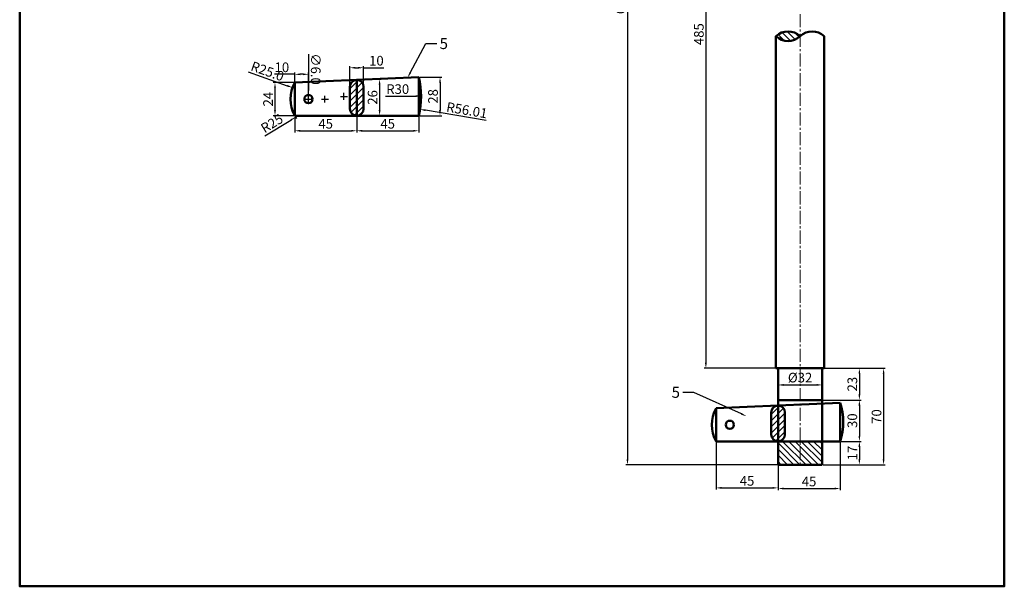
# Model space of a CAD drawing. Units: millimetres. Extents: x -21 to 693, y -570 to 295.
# Tile 1 of 7: x -21 to 693, y -570 to -159. Entities that reach past the tile are written whole.
import ezdxf
from ezdxf import colors
from ezdxf.entities.mleader import LeaderData, LeaderLine
from ezdxf.math import Vec2, Vec3

# ---------------------------------------------------------------- set-up
doc = ezdxf.new("R2010")
doc.units = ezdxf.units.MM
doc.header["$LTSCALE"] = 0.5
doc.linetypes.add('CENTER2', pattern=[28.575, 19.05, -3.175, 3.175, -3.175])
for name, color, linetype, lineweight in [('M-CNTR', 1, 'CENTER2', 18), ('M-DIMS', 2, 'Continuous', 25), ('M-HATC', 8, 'Continuous', 18), ('M-OUTL', 7, 'Continuous', 50), ('M-TEXT', 3, 'Continuous', 25), ('M-TTLB', 7, 'Continuous', 50)]:
    doc.layers.add(name, color=color, linetype=linetype, lineweight=lineweight)
doc.styles.get("Standard").update_dxf_attribs({"font": 'arial.ttf'})
doc.dimstyles.new('ISO-25', dxfattribs={"dimtxt": 7, "dimasz": 4, "dimexe": 1.25, "dimexo": 0.625, "dimtad": 1, "dimdec": 0, "dimtxsty": 'Standard', "dimcen": 2.5, "dimadec": 0, "dimazin": 0, "dimtfac": 1, "dimtdec": 0, "dimtofl": 0, "dimtmove": 0, "dimatfit": 3, "dimfxl": 1, "dimarcsym": 0})

# ---------------------------------------------------------------- blocks, each defined once
blk = doc.blocks.new('*D28')
at = {"layer": 'Defpoints', "color": 0, "ltscale": 0.5, "transparency": 16777216}
for p in [(545.05, 188.11), (419.62, -481.89), (545.05, -481.89)]:
    blk.add_point(p, dxfattribs=at)
at = {"layer": 'M-DIMS', "color": 0, "lineweight": -2, "ltscale": 0.5, "transparency": 16777216}
for p, q in [((544.43, 188.11), (418.37, 188.11)), ((419.62, 184.11), (419.62, -477.89)), ((544.43, -481.89), (418.37, -481.89))]:
    blk.add_line(p, q, dxfattribs=at)
at = {"layer": 'M-DIMS', "color": 0, "ltscale": 0.5, "transparency": 16777216}
for points in [[(418.95, 184.11), (420.29, 184.11), (419.62, 188.11)], [(418.95, -477.89), (420.29, -477.89), (419.62, -481.89)]]:
    blk.add_solid(points, dxfattribs=at)
at = {"layer": 'M-DIMS', "color": 0, "ltscale": 0.5, "transparency": 16777216, "insert": (415.42, -146.89), "char_height": 7, "attachment_point": 5, "rotation": 90}
blk.add_mtext('670', dxfattribs=at)
blk = doc.blocks.new('*D29')
at = {"layer": 'Defpoints', "color": 0, "ltscale": 0.5, "transparency": 16777216}
for p in [(511.59, 73.11), (476.54, -411.89), (528.15, -411.89)]:
    blk.add_point(p, dxfattribs=at)
at = {"layer": 'M-DIMS', "color": 0, "lineweight": -2, "ltscale": 0.5, "transparency": 16777216}
for p, q in [((510.97, 73.11), (475.29, 73.11)), ((476.54, 69.11), (476.54, -407.89)), ((527.53, -411.89), (475.29, -411.89))]:
    blk.add_line(p, q, dxfattribs=at)
at = {"layer": 'M-DIMS', "color": 0, "ltscale": 0.5, "transparency": 16777216}
for points in [[(475.87, 69.11), (477.21, 69.11), (476.54, 73.11)], [(475.87, -407.89), (477.21, -407.89), (476.54, -411.89)]]:
    blk.add_solid(points, dxfattribs=at)
at = {"layer": 'M-DIMS', "color": 0, "ltscale": 0.5, "transparency": 16777216, "insert": (472.34, -169.39), "char_height": 7, "attachment_point": 5, "rotation": 90}
blk.add_mtext('485', dxfattribs=at)
blk = doc.blocks.new('*D31')
at = {"layer": 'Defpoints', "color": 0, "ltscale": 0.5, "transparency": 16777216}
for p in [(528.9, -423.39), (560.9, -423.39), (560.9, -423.95)]:
    blk.add_point(p, dxfattribs=at)
at = {"layer": 'M-DIMS', "color": 0, "lineweight": -2, "ltscale": 0.5, "transparency": 16777216}
for p, q in [((528.9, -424.01), (528.9, -425.2)), ((532.9, -423.95), (556.9, -423.95)), ((560.9, -424.01), (560.9, -425.2))]:
    blk.add_line(p, q, dxfattribs=at)
at = {"layer": 'M-DIMS', "color": 0, "ltscale": 0.5, "transparency": 16777216}
for points in [[(532.9, -423.28), (532.9, -424.61), (528.9, -423.95)], [(556.9, -423.28), (556.9, -424.61), (560.9, -423.95)]]:
    blk.add_solid(points, dxfattribs=at)
at = {"layer": 'M-DIMS', "color": 0, "ltscale": 0.5, "transparency": 16777216, "insert": (544.9, -419.55), "char_height": 7, "attachment_point": 5}
blk.add_mtext('%%C32', dxfattribs=at)
blk = doc.blocks.new('*D32')
at = {"layer": 'Defpoints', "color": 0, "ltscale": 0.5, "transparency": 16777216}
for p in [(560.9, -411.89), (560.9, -481.89), (605.51, -481.89)]:
    blk.add_point(p, dxfattribs=at)
at = {"layer": 'M-DIMS', "color": 0, "lineweight": -2, "ltscale": 0.5, "transparency": 16777216}
for p, q in [((561.53, -411.89), (606.76, -411.89)), ((605.51, -415.89), (605.51, -477.89)), ((561.53, -481.89), (606.76, -481.89))]:
    blk.add_line(p, q, dxfattribs=at)
at = {"layer": 'M-DIMS', "color": 0, "ltscale": 0.5, "transparency": 16777216}
for points in [[(604.84, -415.89), (606.17, -415.89), (605.51, -411.89)], [(604.84, -477.89), (606.17, -477.89), (605.51, -481.89)]]:
    blk.add_solid(points, dxfattribs=at)
at = {"layer": 'M-DIMS', "color": 0, "ltscale": 0.5, "transparency": 16777216, "insert": (601.31, -446.89), "char_height": 7, "attachment_point": 5, "rotation": 90}
blk.add_mtext('70', dxfattribs=at)
blk = doc.blocks.new('*D33')
at = {"layer": 'Defpoints', "color": 0, "ltscale": 0.5, "transparency": 16777216}
for p in [(560.9, -411.89), (560.9, -434.89), (587.93, -434.89)]:
    blk.add_point(p, dxfattribs=at)
at = {"layer": 'M-DIMS', "color": 0, "lineweight": -2, "ltscale": 0.5, "transparency": 16777216}
for p, q in [((561.53, -411.89), (589.18, -411.89)), ((587.93, -415.89), (587.93, -430.89)), ((561.53, -434.89), (589.18, -434.89))]:
    blk.add_line(p, q, dxfattribs=at)
at = {"layer": 'M-DIMS', "color": 0, "ltscale": 0.5, "transparency": 16777216}
for points in [[(587.26, -415.89), (588.6, -415.89), (587.93, -411.89)], [(587.26, -430.89), (588.6, -430.89), (587.93, -434.89)]]:
    blk.add_solid(points, dxfattribs=at)
at = {"layer": 'M-DIMS', "color": 0, "ltscale": 0.5, "transparency": 16777216, "insert": (583.73, -423.39), "char_height": 7, "attachment_point": 5, "rotation": 90}
blk.add_mtext('23', dxfattribs=at)
blk = doc.blocks.new('*D34')
at = {"layer": 'Defpoints', "color": 0, "ltscale": 0.5, "transparency": 16777216}
for p in [(575.35, -434.89), (575.35, -464.89), (587.93, -464.89)]:
    blk.add_point(p, dxfattribs=at)
at = {"layer": 'M-DIMS', "color": 0, "lineweight": -2, "ltscale": 0.5, "transparency": 16777216}
for p, q in [((575.98, -434.89), (589.18, -434.89)), ((587.93, -438.89), (587.93, -460.89)), ((575.98, -464.89), (589.18, -464.89))]:
    blk.add_line(p, q, dxfattribs=at)
at = {"layer": 'M-DIMS', "color": 0, "ltscale": 0.5, "transparency": 16777216}
for points in [[(587.26, -438.89), (588.6, -438.89), (587.93, -434.89)], [(587.26, -460.89), (588.6, -460.89), (587.93, -464.89)]]:
    blk.add_solid(points, dxfattribs=at)
at = {"layer": 'M-DIMS', "color": 0, "ltscale": 0.5, "transparency": 16777216, "insert": (583.73, -449.89), "char_height": 7, "attachment_point": 5, "rotation": 90}
blk.add_mtext('30', dxfattribs=at)
blk = doc.blocks.new('*D35')
at = {"layer": 'Defpoints', "color": 0, "ltscale": 0.5, "transparency": 16777216}
for p in [(573.9, -464.89), (573.9, -481.89), (587.93, -481.89)]:
    blk.add_point(p, dxfattribs=at)
at = {"layer": 'M-DIMS', "color": 0, "lineweight": -2, "ltscale": 0.5, "transparency": 16777216}
for p, q in [((574.53, -464.89), (589.18, -464.89)), ((587.93, -468.89), (587.93, -477.89)), ((574.53, -481.89), (589.18, -481.89))]:
    blk.add_line(p, q, dxfattribs=at)
at = {"layer": 'M-DIMS', "color": 0, "ltscale": 0.5, "transparency": 16777216}
for points in [[(587.26, -468.89), (588.6, -468.89), (587.93, -464.89)], [(587.26, -477.89), (588.6, -477.89), (587.93, -481.89)]]:
    blk.add_solid(points, dxfattribs=at)
at = {"layer": 'M-DIMS', "color": 0, "ltscale": 0.5, "transparency": 16777216, "insert": (583.79, -473.39), "char_height": 7, "attachment_point": 5, "rotation": 90}
blk.add_mtext('17', dxfattribs=at)
blk = doc.blocks.new('*D36')
at = {"layer": 'Defpoints', "color": 0, "ltscale": 0.5, "transparency": 16777216}
for p in [(573.9, -464.89), (528.9, -481.89), (573.9, -499.13)]:
    blk.add_point(p, dxfattribs=at)
at = {"layer": 'M-DIMS', "color": 0, "lineweight": -2, "ltscale": 0.5, "transparency": 16777216}
for p, q in [((573.9, -465.51), (573.9, -500.38)), ((528.9, -482.51), (528.9, -500.38)), ((532.9, -499.13), (569.9, -499.13))]:
    blk.add_line(p, q, dxfattribs=at)
at = {"layer": 'M-DIMS', "color": 0, "ltscale": 0.5, "transparency": 16777216}
for points in [[(532.9, -498.46), (532.9, -499.8), (528.9, -499.13)], [(569.9, -498.46), (569.9, -499.8), (573.9, -499.13)]]:
    blk.add_solid(points, dxfattribs=at)
at = {"layer": 'M-DIMS', "color": 0, "ltscale": 0.5, "transparency": 16777216, "insert": (551.4, -494.94), "char_height": 7, "attachment_point": 5}
blk.add_mtext('45', dxfattribs=at)
blk = doc.blocks.new('*D37')
at = {"layer": 'Defpoints', "color": 0, "ltscale": 0.5, "transparency": 16777216}
for p in [(483.9, -452.89), (528.9, -481.89), (528.9, -498.66)]:
    blk.add_point(p, dxfattribs=at)
at = {"layer": 'M-DIMS', "color": 0, "lineweight": -2, "ltscale": 0.5, "transparency": 16777216}
for p, q in [((483.9, -453.51), (483.9, -499.91)), ((528.9, -482.51), (528.9, -499.91)), ((487.9, -498.66), (524.9, -498.66))]:
    blk.add_line(p, q, dxfattribs=at)
at = {"layer": 'M-DIMS', "color": 0, "ltscale": 0.5, "transparency": 16777216}
for points in [[(487.9, -498), (487.9, -499.33), (483.9, -498.66)], [(524.9, -498), (524.9, -499.33), (528.9, -498.66)]]:
    blk.add_solid(points, dxfattribs=at)
at = {"layer": 'M-DIMS', "color": 0, "ltscale": 0.5, "transparency": 16777216, "insert": (506.4, -494.48), "char_height": 7, "attachment_point": 5}
blk.add_mtext('45', dxfattribs=at)
blk = doc.blocks.new('*D38')
at = {"layer": 'Defpoints', "color": 0, "ltscale": 0.5, "transparency": 16777216}
for p in [(178.09, -204.54), (163.79, -228.54), (178.09, -228.54)]:
    blk.add_point(p, dxfattribs=at)
at = {"layer": 'M-DIMS', "color": 0, "lineweight": -2, "ltscale": 0.5, "transparency": 16777216}
for p, q in [((177.47, -204.54), (162.54, -204.54)), ((163.79, -208.54), (163.79, -224.54)), ((177.47, -228.54), (162.54, -228.54))]:
    blk.add_line(p, q, dxfattribs=at)
at = {"layer": 'M-DIMS', "color": 0, "ltscale": 0.5, "transparency": 16777216}
for points in [[(163.13, -208.54), (164.46, -208.54), (163.79, -204.54)], [(163.13, -224.54), (164.46, -224.54), (163.79, -228.54)]]:
    blk.add_solid(points, dxfattribs=at)
at = {"layer": 'M-DIMS', "color": 0, "ltscale": 0.5, "transparency": 16777216, "insert": (159.66, -216.54), "char_height": 7, "attachment_point": 5, "rotation": 90}
blk.add_mtext('24', dxfattribs=at)
blk = doc.blocks.new('*D39')
at = {"layer": 'Defpoints', "color": 0, "ltscale": 0.5, "transparency": 16777216}
for p in [(228.09, -193.76), (218.09, -211.86), (228.09, -211.86)]:
    blk.add_point(p, dxfattribs=at)
at = {"layer": 'M-DIMS', "color": 0, "lineweight": -2, "ltscale": 0.5, "transparency": 16777216}
for p, q in [((218.09, -211.24), (218.09, -192.51)), ((228.09, -211.24), (228.09, -192.51)), ((222.09, -193.76), (224.09, -193.76)), ((228.09, -193.76), (242.69, -193.76))]:
    blk.add_line(p, q, dxfattribs=at)
at = {"layer": 'M-DIMS', "color": 0, "ltscale": 0.5, "transparency": 16777216}
for points in [[(222.09, -193.09), (222.09, -194.43), (218.09, -193.76)], [(224.09, -193.09), (224.09, -194.43), (228.09, -193.76)]]:
    blk.add_solid(points, dxfattribs=at)
at = {"layer": 'M-DIMS', "color": 0, "ltscale": 0.5, "transparency": 16777216, "insert": (237.39, -189.56), "char_height": 7, "attachment_point": 5}
blk.add_mtext('10', dxfattribs=at)
blk = doc.blocks.new('*D40')
at = {"layer": 'Defpoints', "color": 0, "ltscale": 0.5, "transparency": 16777216}
for p in [(178.09, -228.54), (223.09, -228.54), (223.09, -239.5)]:
    blk.add_point(p, dxfattribs=at)
at = {"layer": 'M-DIMS', "color": 0, "lineweight": -2, "ltscale": 0.5, "transparency": 16777216}
for p, q in [((178.09, -229.17), (178.09, -240.75)), ((223.09, -229.17), (223.09, -240.75)), ((182.09, -239.5), (219.09, -239.5))]:
    blk.add_line(p, q, dxfattribs=at)
at = {"layer": 'M-DIMS', "color": 0, "ltscale": 0.5, "transparency": 16777216}
for points in [[(182.09, -238.84), (182.09, -240.17), (178.09, -239.5)], [(219.09, -238.84), (219.09, -240.17), (223.09, -239.5)]]:
    blk.add_solid(points, dxfattribs=at)
at = {"layer": 'M-DIMS', "color": 0, "ltscale": 0.5, "transparency": 16777216, "insert": (200.59, -235.32), "char_height": 7, "attachment_point": 5}
blk.add_mtext('45', dxfattribs=at)
blk = doc.blocks.new('*D41')
at = {"layer": 'Defpoints', "color": 0, "ltscale": 0.5, "transparency": 16777216}
for p in [(223.09, -228.54), (268.09, -228.54), (268.09, -239.5)]:
    blk.add_point(p, dxfattribs=at)
at = {"layer": 'M-DIMS', "color": 0, "lineweight": -2, "ltscale": 0.5, "transparency": 16777216}
for p, q in [((223.09, -229.17), (223.09, -240.75)), ((268.09, -229.17), (268.09, -240.75)), ((227.09, -239.5), (264.09, -239.5))]:
    blk.add_line(p, q, dxfattribs=at)
at = {"layer": 'M-DIMS', "color": 0, "ltscale": 0.5, "transparency": 16777216}
for points in [[(227.09, -238.84), (227.09, -240.17), (223.09, -239.5)], [(264.09, -238.84), (264.09, -240.17), (268.09, -239.5)]]:
    blk.add_solid(points, dxfattribs=at)
at = {"layer": 'M-DIMS', "color": 0, "ltscale": 0.5, "transparency": 16777216, "insert": (245.59, -235.32), "char_height": 7, "attachment_point": 5}
blk.add_mtext('45', dxfattribs=at)
blk = doc.blocks.new('*D42')
at = {"layer": 'Defpoints', "color": 0, "ltscale": 0.5, "transparency": 16777216}
for p in [(178.09, -198.53), (178.09, -216.54), (188.09, -216.54)]:
    blk.add_point(p, dxfattribs=at)
at = {"layer": 'M-DIMS', "color": 0, "lineweight": -2, "ltscale": 0.5, "transparency": 16777216}
for p, q in [((178.09, -198.53), (163.5, -198.53)), ((178.09, -215.92), (178.09, -197.28)), ((184.09, -198.53), (182.09, -198.53)), ((188.09, -215.92), (188.09, -197.28))]:
    blk.add_line(p, q, dxfattribs=at)
at = {"layer": 'M-DIMS', "color": 0, "ltscale": 0.5, "transparency": 16777216}
for points in [[(182.09, -197.86), (182.09, -199.19), (178.09, -198.53)], [(184.09, -197.86), (184.09, -199.19), (188.09, -198.53)]]:
    blk.add_solid(points, dxfattribs=at)
at = {"layer": 'M-DIMS', "color": 0, "ltscale": 0.5, "transparency": 16777216, "insert": (168.8, -194.33), "char_height": 7, "attachment_point": 5}
blk.add_mtext('10', dxfattribs=at)
blk = doc.blocks.new('*D43')
at = {"layer": 'Defpoints', "color": 0, "ltscale": 0.5, "transparency": 16777216}
for p in [(200.03, -216.54), (178.71, -229.61)]:
    blk.add_point(p, dxfattribs=at)
at = {"layer": 'M-DIMS', "color": 0, "lineweight": -2, "ltscale": 0.5, "transparency": 16777216}
for p, q in [((200.03, -219.04), (200.03, -214.04)), ((197.53, -216.54), (202.53, -216.54)), ((156.52, -243.21), (175.3, -231.7))]:
    blk.add_line(p, q, dxfattribs=at)
blk.add_arc((200.03, -216.54), 25, 210.1178, 214.36901, dxfattribs=at)
at = {"layer": 'M-DIMS', "color": 0, "ltscale": 0.5, "transparency": 16777216}
blk.add_solid([(174.95, -231.13), (175.65, -232.26), (178.71, -229.61)], dxfattribs=at)
at = {"layer": 'M-DIMS', "color": 0, "ltscale": 0.5, "transparency": 16777216, "insert": (162.01, -234.92), "char_height": 7, "attachment_point": 5, "rotation": 31.50422}
blk.add_mtext('R25', dxfattribs=at)
blk = doc.blocks.new('*D44')
at = {"layer": 'Defpoints', "color": 0, "ltscale": 0.5, "transparency": 16777216}
for p in [(269.87, -214.32), (213.86, -214.54)]:
    blk.add_point(p, dxfattribs=at)
at = {"layer": 'M-DIMS', "color": 0, "lineweight": -2, "ltscale": 0.5, "transparency": 16777216}
blk.add_line((243.91, -214.42), (265.87, -214.34), dxfattribs=at)
at = {"layer": 'M-DIMS', "color": 0, "ltscale": 0.5, "transparency": 16777216}
blk.add_solid([(265.87, -213.67), (265.87, -215), (269.87, -214.32)], dxfattribs=at)
at = {"layer": 'M-DIMS', "color": 0, "ltscale": 0.5, "transparency": 16777216, "insert": (252.87, -210.19), "char_height": 7, "attachment_point": 5, "rotation": 0.22564}
blk.add_mtext('R30', dxfattribs=at)
blk = doc.blocks.new('*D45')
at = {"layer": 'Defpoints', "color": 0, "ltscale": 0.5, "transparency": 16777216}
for p in [(234.13, -202.05), (234.13, -228.54), (239.72, -228.54)]:
    blk.add_point(p, dxfattribs=at)
at = {"layer": 'M-DIMS', "color": 0, "lineweight": -2, "ltscale": 0.5, "transparency": 16777216}
for p, q in [((234.76, -202.05), (240.97, -202.05)), ((239.72, -206.05), (239.72, -224.54)), ((234.76, -228.54), (240.97, -228.54))]:
    blk.add_line(p, q, dxfattribs=at)
at = {"layer": 'M-DIMS', "color": 0, "ltscale": 0.5, "transparency": 16777216}
for points in [[(239.05, -206.05), (240.38, -206.05), (239.72, -202.05)], [(239.05, -224.54), (240.38, -224.54), (239.72, -228.54)]]:
    blk.add_solid(points, dxfattribs=at)
at = {"layer": 'M-DIMS', "color": 0, "ltscale": 0.5, "transparency": 16777216, "insert": (235.52, -215.3), "char_height": 7, "attachment_point": 5, "rotation": 90}
blk.add_mtext('26', dxfattribs=at)
blk = doc.blocks.new('*D46')
at = {"layer": 'Defpoints', "color": 0, "ltscale": 0.5, "transparency": 16777216}
for p in [(268.09, -200.54), (268.09, -228.54), (283.57, -228.54)]:
    blk.add_point(p, dxfattribs=at)
at = {"layer": 'M-DIMS', "color": 0, "lineweight": -2, "ltscale": 0.5, "transparency": 16777216}
for p, q in [((268.72, -200.54), (284.82, -200.54)), ((283.57, -204.54), (283.57, -224.54)), ((268.72, -228.54), (284.82, -228.54))]:
    blk.add_line(p, q, dxfattribs=at)
at = {"layer": 'M-DIMS', "color": 0, "ltscale": 0.5, "transparency": 16777216}
for points in [[(282.9, -204.54), (284.24, -204.54), (283.57, -200.54)], [(282.9, -224.54), (284.24, -224.54), (283.57, -228.54)]]:
    blk.add_solid(points, dxfattribs=at)
at = {"layer": 'M-DIMS', "color": 0, "ltscale": 0.5, "transparency": 16777216, "insert": (279.37, -214.54), "char_height": 7, "attachment_point": 5, "rotation": 90}
blk.add_mtext('28', dxfattribs=at)
blk = doc.blocks.new('COTTER-SECTION')
for p, q in [((0, 21), (0, 5)), ((10, 21), (10, 5))]:
    blk.add_line(p, q)
for centre, start, end in [((5, 21), 0, 180), ((5, 5), 180, 0)]:
    blk.add_arc(centre, 5, start, end)
blk = doc.blocks.new('*D65')
at = {"layer": 'Defpoints', "color": 0, "ltscale": 0.5, "transparency": 16777216}
for p in [(176.47, -208.17), (200.03, -216.54)]:
    blk.add_point(p, dxfattribs=at)
at = {"layer": 'M-DIMS', "color": 0, "lineweight": -2, "ltscale": 0.5, "transparency": 16777216}
for p, q in [((144.33, -196.74), (172.7, -206.83)), ((200.03, -219.04), (200.03, -214.04)), ((197.53, -216.54), (202.53, -216.54))]:
    blk.add_line(p, q, dxfattribs=at)
at = {"layer": 'M-DIMS', "color": 0, "ltscale": 0.5, "transparency": 16777216}
blk.add_solid([(172.93, -206.2), (172.48, -207.46), (176.47, -208.17)], dxfattribs=at)
at = {"layer": 'M-DIMS', "color": 0, "ltscale": 0.5, "transparency": 16777216, "insert": (158.04, -197.16), "char_height": 7, "attachment_point": 5, "rotation": 340.4299}
blk.add_mtext('R25.0', dxfattribs=at)
blk = doc.blocks.new('*D66')
at = {"layer": 'Defpoints', "color": 0, "ltscale": 0.5, "transparency": 16777216}
for p in [(213.86, -214.54), (269.08, -223.95)]:
    blk.add_point(p, dxfattribs=at)
at = {"layer": 'M-DIMS', "color": 0, "lineweight": -2, "ltscale": 0.5, "transparency": 16777216}
for p, q in [((213.86, -217.04), (213.86, -212.04)), ((211.36, -214.54), (216.36, -214.54)), ((317.1, -232.12), (273.02, -224.62))]:
    blk.add_line(p, q, dxfattribs=at)
at = {"layer": 'M-DIMS', "color": 0, "ltscale": 0.5, "transparency": 16777216}
blk.add_solid([(273.13, -223.96), (272.91, -225.27), (269.08, -223.95)], dxfattribs=at)
at = {"layer": 'M-DIMS', "color": 0, "ltscale": 0.5, "transparency": 16777216, "insert": (302.91, -225.45), "char_height": 7, "attachment_point": 5, "rotation": 350.33541}
blk.add_mtext('R56.01', dxfattribs=at)
blk = doc.blocks.new('*D67')
at = {"layer": 'Defpoints', "color": 0, "ltscale": 0.5, "transparency": 16777216}
for p in [(188.09, -213.54), (188.1, -219.54)]:
    blk.add_point(p, dxfattribs=at)
at = {"layer": 'M-DIMS', "color": 0, "lineweight": -2, "ltscale": 0.5, "transparency": 16777216}
for p, q in [((188.04, -183.96), (188.08, -209.54)), ((188.09, -219.04), (188.09, -214.04)), ((185.59, -216.54), (190.59, -216.54))]:
    blk.add_line(p, q, dxfattribs=at)
at = {"layer": 'M-DIMS', "color": 0, "ltscale": 0.5, "transparency": 16777216}
blk.add_solid([(188.75, -209.54), (187.42, -209.54), (188.09, -213.54)], dxfattribs=at)
at = {"layer": 'M-DIMS', "color": 0, "ltscale": 0.5, "transparency": 16777216, "insert": (192.45, -194.74), "char_height": 7, "attachment_point": 5, "rotation": 270.09284}
blk.add_mtext('∅6.0', dxfattribs=at)

msp = doc.modelspace()

# ---------------------------------------------------------------- hatches: boundary and pattern name
at = {"layer": 'M-HATC', "ltscale": 0.5}
h = msp.add_hatch(dxfattribs=at)
h.set_pattern_fill('ANSI31', color=256, angle=90)
h.paths.add_polyline_path([(562.403, -136.2127, 0.39671485), (544.903, -136.2127, 0.39671485)])
h.paths.add_polyline_path([(544.903, -170.8866, -0.39671485), (527.403, -170.8866, -0.39671485)])
h.paths.add_polyline_path([(544.903, -464.8866), (528.903, -464.8866), (528.903, -481.8866), (544.903, -481.8866)])
h.paths.add_polyline_path([(560.903, -464.8866), (544.903, -464.8866), (544.903, -481.8866), (560.903, -481.8866)])
at = {"layer": 'M-HATC'}
h = msp.add_hatch(dxfattribs=at)
h.set_pattern_fill('ANSI31', color=256)
h.set_pattern_definition([(45, (-460.5597, 252.7163), (-2.245064, 2.245064), [])])
h.paths.add_polyline_path([(228.0949, -207.5414, 0.41421356), (223.0949, -202.5414), (223.0949, -228.5414, 0.41421356), (228.0949, -223.5414)])
h.paths.add_polyline_path([(223.0949, -202.5414), (222.6514, -202.5611, 0.38842868), (218.0949, -207.5414), (218.0949, -223.5414, 0.41421356), (223.0949, -228.5414)])
h = msp.add_hatch(dxfattribs=at)
h.set_pattern_fill('ANSI31', color=256)
h.set_pattern_definition([(45, (-154.7516, 16.371), (-2.245064, 2.245064), [])])
h.paths.add_polyline_path([(533.903, -443.8866, 0.41421356), (528.903, -438.8866), (528.903, -464.8866, 0.41421356), (533.903, -459.8866)])
h.paths.add_polyline_path([(528.903, -438.8866), (528.4595, -438.9064, 0.38842868), (523.903, -443.8866), (523.903, -459.8866, 0.41421356), (528.903, -464.8866)])

# ---------------------------------------------------------------- linework, layer by layer
at = {"layer": 'M-CNTR'}
msp.add_line((544.903, 188.1134), (544.903, -481.8866), dxfattribs=at)
at = {"layer": 'M-OUTL'}
for p, q in [((527.403, -411.8866), (527.403, -170.8866)), ((562.403, -411.8866), (562.403, -170.8866)), ((268.0949, -200.5414), (178.0949, -204.5414)), ((178.0949, -204.5414), (178.0949, -228.5414)), ((223.0949, -202.5414), (223.0949, -228.5414)), ((268.0949, -228.5414), (268.0949, -200.5414)), ((178.0949, -228.5414), (268.0949, -228.5414)), ((528.903, -411.8866), (527.403, -411.8866)), ((528.903, -434.8866), (528.903, -411.8866)), ((560.903, -411.8866), (528.903, -411.8866)), ((560.903, -434.8866), (560.903, -411.8866)), ((560.903, -411.8866), (562.403, -411.8866)), ((528.903, -434.8866), (528.903, -464.8866)), ((560.903, -434.8866), (528.903, -434.8866)), ((560.903, -481.8866), (560.903, -434.8866)), ((573.903, -436.8866), (483.903, -440.8866)), ((483.903, -440.8866), (483.903, -464.8866)), ((573.903, -464.8866), (573.903, -436.8866)), ((483.903, -464.8866), (573.903, -464.8866)), ((560.903, -464.8866), (528.903, -464.8866)), ((528.903, -464.8866), (528.903, -481.8866)), ((528.903, -481.8866), (560.903, -481.8866))]:
    msp.add_line(p, q, dxfattribs=at)
for centre in [(188.0949, -216.5414), (493.903, -452.8866)]:
    msp.add_circle(centre, 3, dxfattribs=at)
for centre, radius, start, end in [((536.153, -180.1791), 12.7637, 46.7220744, 133.2779256), ((536.153, -161.5942), 12.7637, 226.7220744, 313.2779256), ((553.653, -180.1791), 12.7637, 46.7220643, 133.2779256), ((200.0266, -216.5414), 25, 151.314598, 208.685402), ((505.8347, -452.8866), 25, 151.314598, 208.685402), ((533.1751, -450.8866), 43.067, 341.0298835, 18.9701165)]:
    msp.add_arc(centre, radius, start, end, dxfattribs=at)
at = {"layer": 'M-OUTL', "ltscale": 0.5}
msp.add_arc((213.8581, -214.5414), 56.0146, 345.526338, 14.473662, dxfattribs=at)
at = {"layer": 'M-TTLB', "ltscale": 0.5}
msp.add_lwpolyline([(-21.49, 295.4176), (693.1139, 295.4176), (693.1139, -570.0874), (-21.49, -570.0874)], close=True, dxfattribs=at)

# ---------------------------------------------------------------- block references
at = {"layer": 'M-OUTL'}
for p in [(218.095, -228.541), (523.9031, -464.8863)]:
    msp.add_blockref('COTTER-SECTION', p, dxfattribs=at)

# ---------------------------------------------------------------- dimensions: what is measured, and where the dimension line sits
at = {"layer": 'M-DIMS', "ltscale": 0.5}
for base, p1, p2, picture, middle in [((419.6197, -481.8866), (545.0534, 188.1134), (545.0534, -481.8866), '*D28', (415.4207, -146.8866)), ((476.5413, -411.8866), (511.5903, 73.1134), (528.153, -411.8866), '*D29', (472.3422, -169.3866)), ((163.7946, -228.5414), (178.0949, -204.5414), (178.0949, -228.5414), '*D38', (159.6553, -216.5414)), ((239.7165, -228.5414), (234.1312, -202.0509), (234.1312, -228.5414), '*D45', (235.5175, -215.2961)), ((283.5693, -228.5414), (268.0949, -200.5414), (268.0949, -228.5414), '*D46', (279.3703, -214.5414)), ((605.5057, -481.8866), (560.903, -411.8866), (560.903, -481.8866), '*D32', (601.3067, -446.8866)), ((587.9296, -434.8866), (560.903, -411.8866), (560.903, -434.8866), '*D33', (583.7282, -423.3866)), ((587.9296, -464.8866), (575.3538, -434.8866), (575.3538, -464.8866), '*D34', (583.7282, -449.8866)), ((587.9296, -481.8866), (573.903, -464.8866), (573.903, -481.8866), '*D35', (583.7903, -473.3866))]:
    dim = msp.add_linear_dim(base=base, p1=p1, p2=p2, angle=90, dimstyle='ISO-25', override={"dimclrd": 0, "dimclre": 0, "dimclrt": 0}, dxfattribs=at)
    dim.commit()
    dim.dimension.update_dxf_attribs({"geometry": picture, "text_midpoint": middle})
dim = msp.add_diameter_dim_2p(p1=(188.0998, -219.5414), p2=(188.0901, -213.5414), dimstyle='ISO-25', override={"dimdec": 1, "dimlfac": 1, "dimrnd": 0, "dimzin": 0, "dimdsep": 46, "dimlunit": 2}, dxfattribs=at)
dim.commit()
dim.dimension.update_dxf_attribs({"geometry": '*D67', "text_midpoint": (188.0596, -194.7483), "dimtype": 163})
for base, p1, p2, picture, middle in [((228.0949, -193.7583), (218.0949, -211.8601), (228.0949, -211.8601), '*D39', (237.3922, -189.5593)), ((178.0949, -198.5282), (188.0949, -216.5414), (178.0949, -216.5414), '*D42', (168.7977, -194.3292)), ((223.0949, -239.5046), (178.0949, -228.5414), (223.0949, -228.5414), '*D40', (200.5949, -235.3199)), ((268.0949, -239.5046), (223.0949, -228.5414), (268.0949, -228.5414), '*D41', (245.5949, -235.3199)), ((528.903, -498.6629), (483.903, -452.8866), (528.903, -481.8866), '*D37', (506.403, -494.4782)), ((573.903, -499.1289), (528.903, -481.8866), (573.903, -464.8866), '*D36', (551.403, -494.9442))]:
    dim = msp.add_linear_dim(base=base, p1=p1, p2=p2, dimstyle='ISO-25', override={"dimclrd": 0, "dimclre": 0, "dimclrt": 0}, dxfattribs=at)
    dim.commit()
    dim.dimension.update_dxf_attribs({"geometry": picture, "text_midpoint": middle})
for mpoint, override, picture, middle in [((176.4708, -208.1674), {"dimdec": 1, "dimlfac": 1, "dimrnd": 0, "dimzin": 0, "dimdsep": 46, "dimlunit": 2}, '*D65', (158.0395, -197.1587)), ((178.7116, -229.6054), {"dimclrd": 0, "dimclre": 0, "dimclrt": 0}, '*D43', (162.0108, -234.9164))]:
    dim = msp.add_radius_dim(center=(200.0266, -216.5414), mpoint=mpoint, dimstyle='ISO-25', override=override, dxfattribs=at)
    dim.commit()
    dim.dimension.update_dxf_attribs({"geometry": picture, "text_midpoint": middle})
dim = msp.add_radius_dim(center=(213.8581, -214.5414), mpoint=(269.8722, -214.3208), text='R30', dimstyle='ISO-25', override={"dimclrd": 0, "dimclre": 0, "dimclrt": 0}, dxfattribs=at)
dim.commit()
dim.dimension.update_dxf_attribs({"geometry": '*D44', "text_midpoint": (252.8865, -214.3877), "dimtype": 164})
dim = msp.add_radius_dim(center=(213.8581, -214.5414), mpoint=(269.0777, -223.9451), dimstyle='ISO-25', override={"dimdec": 2, "dimlfac": 1, "dimrnd": 0, "dimzin": 0, "dimdsep": 46, "dimlunit": 2}, dxfattribs=at)
dim.commit()
dim.dimension.update_dxf_attribs({"geometry": '*D66', "text_midpoint": (302.2094, -229.5874), "dimtype": 164})
dim = msp.add_linear_dim(base=(560.903, -423.9483), p1=(528.903, -423.3866), p2=(560.903, -423.3866), text='%%C<>', dimstyle='ISO-25', override={"dimclrd": 0, "dimclre": 0, "dimclrt": 0}, dxfattribs=at)
dim.commit()
dim.dimension.update_dxf_attribs({"geometry": '*D31', "text_midpoint": (544.903, -419.5535)})

# ---------------------------------------------------------------- leaders
at = {"layer": 'M-TEXT', "ltscale": 0.5}
ml = msp.add_multileader_mtext('Standard', dxfattribs=at)
ml.set_content('5', color=256)
ml.set_leader_properties()
ml.build(insert=Vec2(0, 0))
ctx = ml.context
ctx.base_point, ctx.char_height, ctx.plane_origin = Vec3(281.2821, -176.2713), 8, Vec3(260.0915, -200.8971)
notes = []
notes.append((ctx, [(0, (1, 1, 0), (273.2821, -176.2713), (1, 0), 8, [(0, [(260.0915, -200.8971)], 0, [])])]))
ctx.mtext.insert, ctx.mtext.flow_direction = Vec3(283.2821, -172.2031), 5
ml = msp.add_multileader_mtext('Standard', dxfattribs=at)
ml.set_content('5', color=256)
ml.set_leader_properties()
ml.build(insert=Vec2(0, 0))
ctx = ml.context
ctx.base_point, ctx.char_height, ctx.plane_origin = Vec3(450.3992, -429.376), 8, Vec3(505.9792, -446.6518)
ctx.text_align_type = 2
notes.append((ctx, [(0, (1, 1, 0), (467.7035, -429.376), (-1, 0), 8, [(0, [(505.9792, -446.6518)], 0, [])])]))
ctx.mtext.insert, ctx.mtext.alignment, ctx.mtext.flow_direction = Vec3(457.7035, -425.3078), 3, 5
for ctx, leaders in notes:
    for number, flags, end, landing, length, lines in leaders:
        leader = LeaderData()
        leader.index, (leader.has_last_leader_line, leader.has_dogleg_vector, leader.attachment_direction) = number, flags
        leader.last_leader_point, leader.dogleg_vector, leader.dogleg_length = Vec3(end), Vec3(landing), length
        for number, points, colour, breaks in lines:
            line = LeaderLine()
            line.index, line.vertices, line.color, line.breaks = number, Vec3.list(points), colors.encode_raw_color(colour), breaks
            leader.lines.append(line)
        ctx.leaders.append(leader)

doc.saveas('drawing.dxf')
